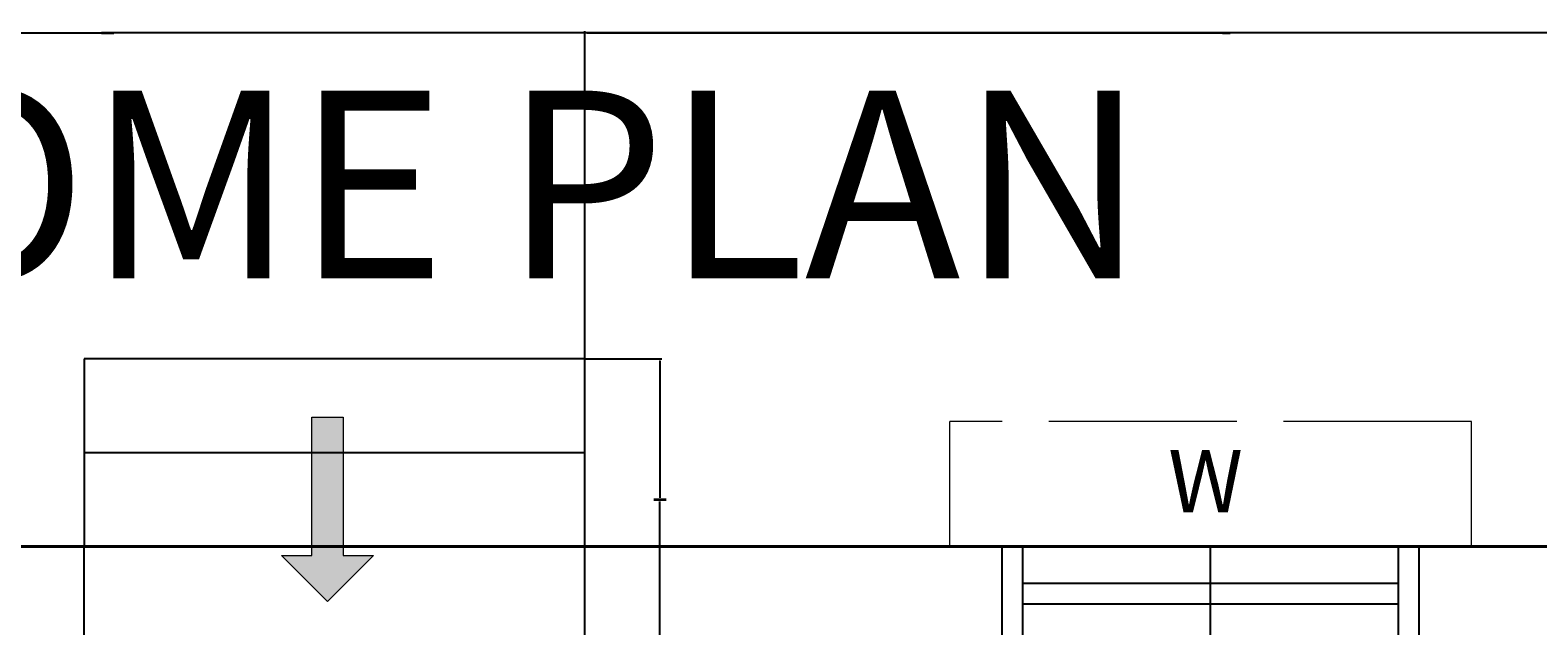
# Model space of a CAD drawing. Units: inches. Extents: x -301 to 715, y -607 to 364.
# Tile 119 of 141: x -43 to 101, y 303 to 360. Entities that reach past the tile are written whole.
import ezdxf

# ---------------------------------------------------------------- set-up
doc = ezdxf.new("R2010")
doc.units = ezdxf.units.IN
doc.header["$MEASUREMENT"] = 0
doc.linetypes.add('ACAD_ISO02W100', pattern=[15, 12, -3])
for name, color, linetype, lineweight in [('A-ANNO-DIMS', 2, 'Continuous', 18), ('A-ANNO-SYMB', 4, 'Continuous', 18), ('A-ANNO-TEXT', 4, 'Continuous', 18), ('A-ANNO-TITL', 1, 'Continuous', 35), ('A-FLOR-STRS', 2, 'Continuous', 25), ('A-GLAZ', 2, 'Continuous', 25), ('A-GLAZ-OVHD', 2, 'ACAD_ISO02W100', 18), ('A-WALL', 3, 'Continuous', 40)]:
    doc.layers.add(name, color=color, linetype=linetype, lineweight=lineweight)
doc.styles.get("Standard").update_dxf_attribs({"font": 'arial.ttf'})
doc.dimstyles.get("Standard").update_dxf_attribs({"dimtxt": 0.18, "dimasz": 0.18, "dimexe": 0.18, "dimexo": 0.0625, "dimgap": 0.09, "dimtad": 0, "dimtih": 1, "dimtoh": 1, "dimdec": 1, "dimzin": 0, "dimdsep": 46, "dimlunit": 4, "dimtxsty": 'Standard', "dimcen": 0.09, "dimclrd": 3, "dimclre": 4, "dimclrt": 6, "dimadec": 0, "dimazin": 0, "dimtfac": 1, "dimtdec": 1, "dimtofl": 0, "dimtmove": 0, "dimatfit": 3, "dimfxl": 1, "dimtfill": 2, "dimtfillclr": 51, "dimtolj": 1, "dimtzin": 0, "dimarcsym": 0})

# ---------------------------------------------------------------- blocks, each defined once
blk = doc.blocks.new('*U28')
h = blk.add_hatch(color=0)
h.set_gradient(color1=(0, 0, 255), rotation=180, tint=1)
h.paths.add_polyline_path([(0, 0), (-0.25, -0.25), (-0.25, -0.085), (-1, -0.085), (-1, 0.085), (-0.25, 0.085), (-0.25, 0.25)])
at = {"color": 0}
blk.add_lwpolyline([(0, 0), (-0.25, -0.25), (-0.25, -0.085), (-1, -0.085), (-1, 0.085), (-0.25, 0.085), (-0.25, 0.25)], close=True, dxfattribs=at)
blk = doc.blocks.new('WIN-36-PLAN')
for p, q in [((0, 0), (0, 9)), ((2, 0), (2, 9)), ((20, 0), (20, 9)), ((38, 0), (38, 9)), ((40, 0), (40, 9)), ((2, 5.5), (38, 5.5)), ((2, 3.5), (38, 3.5))]:
    blk.add_line(p, q)
blk = doc.blocks.new('WIN-SHADE-50')
at = {"ltscale": 1.5}
for p, q in [((0, 0), (0, 12)), ((50, 12), (0, 12)), ((50, 0), (50, 12)), ((5, 0), (0, 0)), ((45, 0), (50, 0))]:
    blk.add_line(p, q, dxfattribs=at)
blk = doc.blocks.new('ENTRY-STEPS-48')
for p, q in [((0, 27), (0, 18)), ((48, 27), (48, 18)), ((0, 18), (0, 9)), ((48, 9), (48, 18)), ((0, 9), (48, 9)), ((0, 9), (0, 0)), ((48, 0), (48, 9)), ((0, 0), (48, 0))]:
    blk.add_line(p, q)
blk = doc.blocks.new('*D123')
at = {"layer": 'A-ANNO-DIMS', "color": 4, "lineweight": -2, "transparency": 16777216}
for p, q in [((9.96, 328.18), (17.28, 328.18)), ((9.96, 301.18), (17.28, 301.18))]:
    blk.add_line(p, q, dxfattribs=at)
at = {"layer": 'A-ANNO-DIMS', "color": 3, "lineweight": -2, "transparency": 16777216}
for p, q in [((17.1, 328), (17.1, 314.86)), ((17.1, 301.36), (17.1, 314.5))]:
    blk.add_line(p, q, dxfattribs=at)
at = {"layer": 'A-ANNO-DIMS', "color": 3, "transparency": 16777216}
for points in [[(17.07, 328), (17.13, 328), (17.1, 328.18)], [(17.07, 301.36), (17.13, 301.36), (17.1, 301.18)]]:
    blk.add_solid(points, dxfattribs=at)
at = {"layer": 'Defpoints', "color": 0, "transparency": 16777216}
for p in [(9.9, 328.18), (9.9, 301.18), (17.1, 301.18)]:
    blk.add_point(p, dxfattribs=at)
at = {"layer": 'A-ANNO-DIMS', "color": 6, "transparency": 16777216, "insert": (17.1, 314.68), "char_height": 0.18, "attachment_point": 5, "bg_fill": 1, "box_fill_scale": 1.25, "bg_fill_color": 51, "bg_fill_transparency": 0}
blk.add_mtext('\\A1;2\'-3" TYP.', dxfattribs=at)
blk = doc.blocks.new('*D144')
at = {"layer": 'A-ANNO-DIMS', "color": 4, "lineweight": -2, "transparency": 16777216}
for p, q in [((-204.6, 310.24), (-204.6, 359.61)), ((132.9, 310.24), (132.9, 359.61))]:
    blk.add_line(p, q, dxfattribs=at)
at = {"layer": 'A-ANNO-DIMS', "color": 3, "lineweight": -2, "transparency": 16777216}
for p, q in [((-204.42, 359.43), (-36.46, 359.43)), ((132.72, 359.43), (-35.24, 359.43))]:
    blk.add_line(p, q, dxfattribs=at)
at = {"layer": 'A-ANNO-DIMS', "color": 3, "transparency": 16777216}
for points in [[(-204.42, 359.46), (-204.42, 359.4), (-204.6, 359.43)], [(132.72, 359.46), (132.72, 359.4), (132.9, 359.43)]]:
    blk.add_solid(points, dxfattribs=at)
at = {"layer": 'Defpoints', "color": 0, "transparency": 16777216}
for p in [(132.9, 359.43), (-204.6, 310.18), (132.9, 310.18)]:
    blk.add_point(p, dxfattribs=at)
at = {"layer": 'A-ANNO-DIMS', "color": 6, "transparency": 16777216, "insert": (-35.85, 359.43), "char_height": 0.18, "attachment_point": 5, "bg_fill": 1, "box_fill_scale": 1.25, "bg_fill_color": 51, "bg_fill_transparency": 0}
blk.add_mtext('\\A1;28\'-1 1/2"', dxfattribs=at)
blk = doc.blocks.new('*D154')
at = {"layer": 'A-ANNO-DIMS', "color": 4, "lineweight": -2, "transparency": 16777216}
for p, q in [((9.9, 310.24), (9.9, 359.61)), ((132.9, 310.24), (132.9, 359.61))]:
    blk.add_line(p, q, dxfattribs=at)
at = {"layer": 'A-ANNO-DIMS', "color": 3, "lineweight": -2, "transparency": 16777216}
for p, q in [((10.08, 359.43), (71.01, 359.43)), ((132.72, 359.43), (71.79, 359.43))]:
    blk.add_line(p, q, dxfattribs=at)
at = {"layer": 'A-ANNO-DIMS', "color": 3, "transparency": 16777216}
for points in [[(10.08, 359.46), (10.08, 359.4), (9.9, 359.43)], [(132.72, 359.46), (132.72, 359.4), (132.9, 359.43)]]:
    blk.add_solid(points, dxfattribs=at)
at = {"layer": 'Defpoints', "color": 0, "transparency": 16777216}
for p in [(132.9, 359.43), (9.9, 310.18), (132.9, 310.18)]:
    blk.add_point(p, dxfattribs=at)
at = {"layer": 'A-ANNO-DIMS', "color": 6, "transparency": 16777216, "insert": (71.4, 359.43), "char_height": 0.18, "attachment_point": 5, "bg_fill": 1, "box_fill_scale": 1.25, "bg_fill_color": 51, "bg_fill_transparency": 0}
blk.add_mtext('\\A1;10\'-3"', dxfattribs=at)

msp = doc.modelspace()

# ---------------------------------------------------------------- linework, layer by layer
at = {"layer": 'A-WALL'}
msp.add_line((132.9, 310.18), (-204.6, 310.18), dxfattribs=at)

# ---------------------------------------------------------------- block references
at = {"layer": 'A-ANNO-SYMB', "xscale": 17.68611049110349, "yscale": 17.68611049110349, "zscale": 17.68611049110349, "rotation": 270}
msp.add_blockref('*U28', (-14.77, 304.91), dxfattribs=at)
at = {"layer": 'A-FLOR-STRS', "rotation": 180}
msp.add_blockref('ENTRY-STEPS-48', (9.9, 328.18), dxfattribs=at)
at = {"layer": 'A-GLAZ'}
msp.add_blockref('WIN-36-PLAN', (49.9, 301.18), dxfattribs=at)
at = {"layer": 'A-GLAZ-OVHD'}
msp.add_blockref('WIN-SHADE-50', (44.9, 310.18), dxfattribs=at)

# ---------------------------------------------------------------- texts
at = {"layer": 'A-ANNO-TEXT'}
msp.add_text('W', height=6, dxfattribs=at).set_placement((65.82, 313.45))
at = {"layer": 'A-ANNO-TITL'}
msp.add_text('3BHK HOME PLAN', height=18, dxfattribs=at).set_placement((-142.9, 335.91))

# ---------------------------------------------------------------- dimensions: what is measured, and where the dimension line sits
at = {"layer": 'A-ANNO-DIMS'}
for p1, picture, middle in [((-204.6, 310.18), '*D144', (-35.85, 359.43)), ((9.9, 310.18), '*D154', (71.4, 359.43))]:
    dim = msp.add_linear_dim(base=(132.9, 359.43), p1=p1, p2=(132.9, 310.18), dimstyle='Standard', override={"dimdec": 1, "dimlfac": 1, "dimrnd": 0, "dimzin": 1, "dimdsep": 46, "dimlunit": 4, "dimfrac": 2}, dxfattribs=at)
    dim.commit()
    dim.dimension.update_dxf_attribs({"geometry": picture, "text_midpoint": middle})
dim = msp.add_linear_dim(base=(17.1, 301.18), p1=(9.9, 328.18), p2=(9.9, 301.18), angle=270, text='<> TYP.', dimstyle='Standard', override={"dimdec": 1, "dimlfac": 1, "dimrnd": 0, "dimzin": 1, "dimdsep": 46, "dimlunit": 4, "dimfrac": 2}, dxfattribs=at)
dim.commit()
dim.dimension.update_dxf_attribs({"geometry": '*D123', "text_midpoint": (17.1, 314.68)})

doc.saveas('drawing.dxf')
